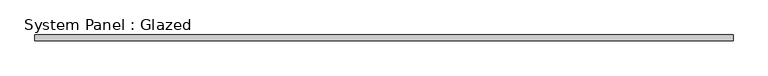
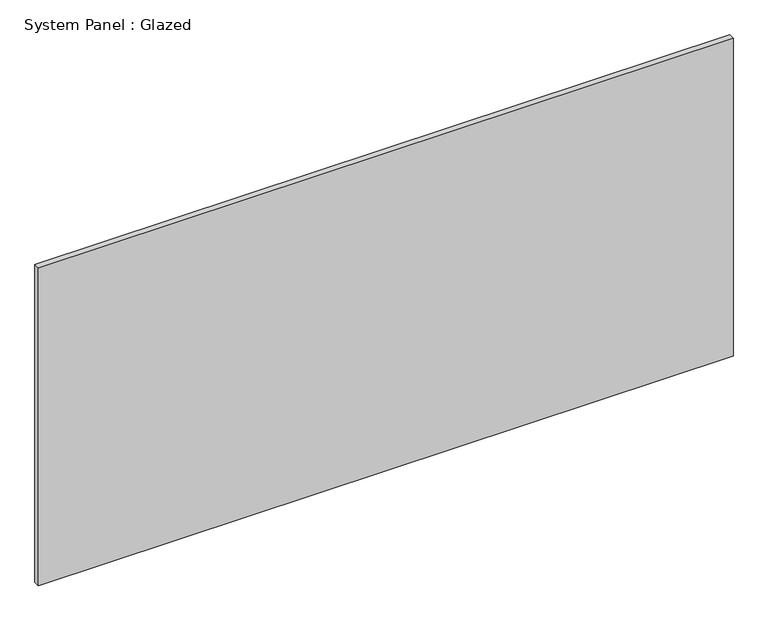
"""IFC4 building model written with IfcOpenShell, lengths in millimetres: plate geometry, System Panel : Glazed."""

from ifc_helpers import new_model, si_unit, origin, origin_with_axes, place, context, project, spatial, polyline, outline, extrude, source, transform, mapped, element, save


def system_panel_glazed_37f15d2e(model_context):
    return source(origin(), model_context, "Body", "SweptSolid", [
        extrude(outline(polyline([(1476.3750002, 19.05), (-1476.3750002, 19.05), (-1476.3750002, 44.45), (1476.3750002, 44.45), (1476.3750002, 19.05)])), origin_with_axes(), (0.0, 0.0, 1.0), 1428.75),
    ])


if __name__ == "__main__":
    model = new_model("IFC4")
    model_context = context("Model", 3, world=origin())
    ifc_project = project(units=[si_unit("LENGTHUNIT", "METRE", prefix="MILLI")], contexts=[model_context])
    site = spatial("IfcSite", under=ifc_project)
    building = spatial("IfcBuilding", under=site)
    placement = place(None, origin())
    system_panel_glazed_shape = system_panel_glazed_37f15d2e(model_context)
    element("IfcPlate", 1, ObjectType="System Panel : Glazed", at=placement, inside=building, context=model_context, shape_type="MappedRepresentation", body=[
        mapped(system_panel_glazed_shape, transform((0.0, 0.0, 0.0), x_axis=(1.0, 0.0, 0.0), y_axis=(0.0, 1.0, 0.0), z_axis=(0.0, 0.0, 1.0))),
    ])
    save(model, "model.ifc")

# Revit data of these elements
# Type "System Panel : Glazed"
#   Construction Type Id = "GSP4R"
#   Analytic Construction = "1/8 in Pilkington single glazing"
#   Visual Light Transmittance = 0.9
#   Solar Heat Gain Coefficient = 0.86
#   Heat Transfer Coefficient (U) = 1.18115 BTU/(h·ft²·°F)
#   Define Thermal Properties by = 1
# Element 1 (IfcPlate, "System Panel : Glazed")
#   Materials on its faces: "Glass"
# Materials
#   "Glass": class "Glass", colour RGB 0 128 192, transparency 0.75, Description = "Soda Lime Glass", Cost = 0
